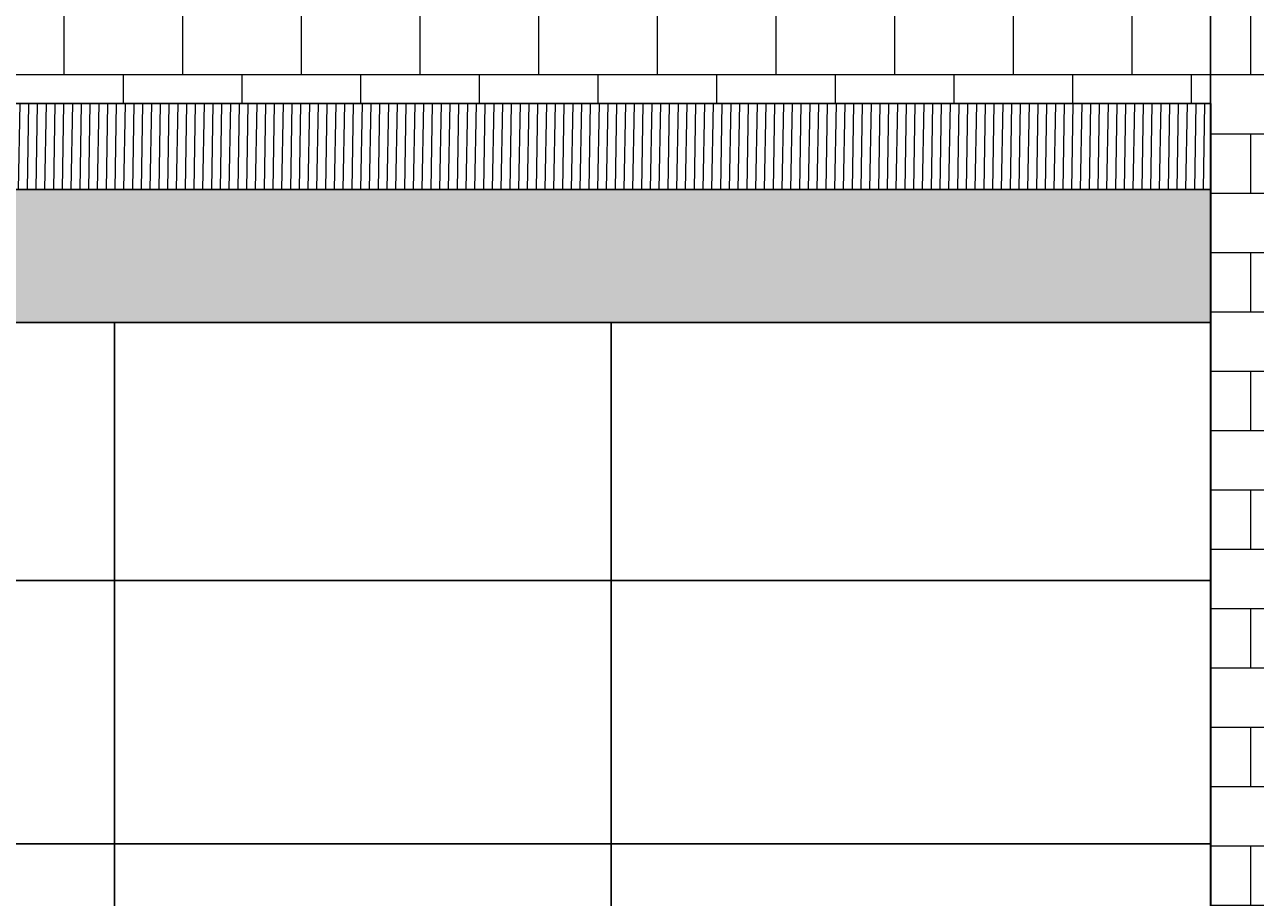
# Model space of a CAD drawing. Units: inches. Extents: x -26 to 776, y -22 to 650.
# Tile 6 of 62: x 98 to 222, y 67 to 155. Entities that reach past the tile are written whole.
import ezdxf

# ---------------------------------------------------------------- set-up
doc = ezdxf.new("R2010")
doc.units = ezdxf.units.IN
doc.header["$MEASUREMENT"] = 0
for name, color, linetype, lineweight in [('A-ANNO-DIMS', 2, 'Continuous', 18), ('A-DETL-PATT', 8, 'Continuous', 13), ('A-DOOR', 3, 'Continuous', 25), ('A-DOOR-PATT', 8, 'Continuous', 13), ('A-WALL-PATT', 8, 'Continuous', 13)]:
    doc.layers.add(name, color=color, linetype=linetype, lineweight=lineweight)
doc.styles.get("Standard").update_dxf_attribs({"font": 'arial.ttf'})
doc.dimstyles.get("Standard").update_dxf_attribs({"dimtxt": 0.5625, "dimasz": 0.18, "dimexe": 0.18, "dimexo": 0.0625, "dimgap": 0.09, "dimtad": 0, "dimtih": 1, "dimtoh": 1, "dimdec": 4, "dimzin": 0, "dimdsep": 46, "dimlunit": 4, "dimtxsty": 'Standard', "dimcen": 0.09, "dimadec": 0, "dimazin": 0, "dimtfac": 1, "dimtdec": 4, "dimtofl": 0, "dimtmove": 0, "dimatfit": 3, "dimfxl": 1, "dimtolj": 1, "dimtzin": 0, "dimarcsym": 0})

# ---------------------------------------------------------------- blocks, each defined once
blk = doc.blocks.new('*D14')
at = {"layer": 'A-ANNO-DIMS', "color": 0, "lineweight": -2, "transparency": 16777216}
for p, q in [((191.62, 613.27), (-25.48, 613.27)), ((-25.3, 613.09), (-25.3, 314.75)), ((-25.3, 15.66), (-25.3, 314)), ((11.04, 15.48), (-25.48, 15.48))]:
    blk.add_line(p, q, dxfattribs=at)
at = {"layer": 'A-ANNO-DIMS', "color": 0, "transparency": 16777216}
for points in [[(-25.33, 613.09), (-25.27, 613.09), (-25.3, 613.27)], [(-25.33, 15.66), (-25.27, 15.66), (-25.3, 15.48)]]:
    blk.add_solid(points, dxfattribs=at)
at = {"layer": 'Defpoints', "color": 0, "transparency": 16777216}
for p in [(-25.3, 613.27), (191.68, 613.27), (11.11, 15.48)]:
    blk.add_point(p, dxfattribs=at)
at = {"layer": 'A-ANNO-DIMS', "color": 0, "transparency": 16777216, "insert": (-25.3, 314.38), "char_height": 0.562, "attachment_point": 5}
blk.add_mtext('\\A1;597.8', dxfattribs=at)
blk = doc.blocks.new('*D22')
at = {"layer": 'A-ANNO-DIMS', "color": 0, "lineweight": -2, "transparency": 16777216}
for p, q in [((22.89, 15.33), (22.89, 649.86)), ((217.95, 15.54), (217.95, 649.86)), ((23.07, 649.68), (119.19, 649.68)), ((217.77, 649.68), (121.65, 649.68))]:
    blk.add_line(p, q, dxfattribs=at)
at = {"layer": 'A-ANNO-DIMS', "color": 0, "transparency": 16777216}
for points in [[(23.07, 649.71), (23.07, 649.65), (22.89, 649.68)], [(217.77, 649.71), (217.77, 649.65), (217.95, 649.68)]]:
    blk.add_solid(points, dxfattribs=at)
at = {"layer": 'Defpoints', "color": 0, "transparency": 16777216}
for p in [(217.95, 649.68), (22.89, 15.27), (217.95, 15.48)]:
    blk.add_point(p, dxfattribs=at)
at = {"layer": 'A-ANNO-DIMS', "color": 0, "transparency": 16777216, "insert": (120.42, 649.68), "char_height": 0.562, "attachment_point": 5}
blk.add_mtext('\\A1;195.06', dxfattribs=at)
blk = doc.blocks.new('*D37')
at = {"layer": 'A-ANNO-DIMS', "color": 0, "lineweight": -2, "transparency": 16777216}
for p, q in [((231.36, 159.48), (-25.48, 159.48)), ((-25.3, 159.3), (-25.3, 87.85)), ((-25.3, 15.66), (-25.3, 87.11)), ((217.89, 15.48), (-25.48, 15.48))]:
    blk.add_line(p, q, dxfattribs=at)
at = {"layer": 'A-ANNO-DIMS', "color": 0, "transparency": 16777216}
for points in [[(-25.33, 159.3), (-25.27, 159.3), (-25.3, 159.48)], [(-25.33, 15.66), (-25.27, 15.66), (-25.3, 15.48)]]:
    blk.add_solid(points, dxfattribs=at)
at = {"layer": 'Defpoints', "color": 0, "transparency": 16777216}
for p in [(-25.3, 159.48), (231.42, 159.48), (217.95, 15.48)]:
    blk.add_point(p, dxfattribs=at)
at = {"layer": 'A-ANNO-DIMS', "color": 0, "transparency": 16777216, "insert": (-25.3, 87.48), "char_height": 0.562, "attachment_point": 5}
blk.add_mtext('\\A1;144', dxfattribs=at)

msp = doc.modelspace()

# ---------------------------------------------------------------- hatches: boundary and pattern name
at = {"layer": 'A-DETL-PATT'}
h = msp.add_hatch(dxfattribs=at)
h.set_pattern_fill('ANSI31', color=256, scale=7.1, angle=44)
h.paths.add_polyline_path([(231.4249, 197.3298), (216.1056, 197.3298), (216.1056, 159.4824), (231.4249, 159.4824)])
h.paths.add_polyline_path([(236.4647, 197.3298), (231.4249, 197.3298), (231.4249, 159.4824), (276.1134, 159.4824), (276.1134, 171.4173), (236.4647, 171.4173)])
h.paths.add_polyline_path([(259.7413, 197.3298), (236.4647, 197.3298), (236.4647, 171.4173), (259.7413, 171.4173)], flags=17)
h.paths.add_polyline_path([(276.1134, 197.3298), (261.7413, 197.3298), (261.7413, 171.4173), (276.1134, 171.4173)], flags=17)
h.paths.add_polyline_path([(217.9529, 147.0781), (22.8891, 147.0781), (22.8891, 138.3844), (217.9529, 138.3844)])
h.paths.add_polyline_path([(285.0179, 152.3087), (285.0179, 159.4824), (231.4249, 159.4824), (240.1654, 144.8359), (280.6173, 144.8359)])
h.paths.add_polyline_path([(280.6173, 144.8359), (240.1654, 144.8359), (240.1654, 26.4239), (280.6173, 26.4239)])
h.paths.add_polyline_path([(274.6644, 134.8811), (274.6644, 34.0885), (245.7207, 34.0885), (245.7207, 134.8811)], flags=16)
h.paths.add_polyline_path([(285.0179, 303.3046), (236.4647, 303.3046), (236.4647, 294.4171), (285.0179, 294.4171)])
h.paths.add_polyline_path([(285.0179, 446.0063), (236.4647, 446.0063), (236.4647, 437.1188), (285.0179, 437.1188)])
at = {"layer": 'A-DOOR-PATT'}
h = msp.add_hatch(color=256, dxfattribs=at)
h.dxf.hatch_style = 1
h.paths.add_polyline_path([(217.9529, 138.3844), (22.8891, 138.3844), (22.8891, 124.9232), (217.9529, 124.9232)])
h.paths.add_polyline_path([(274.6644, 134.8811), (245.7207, 134.8811), (245.7207, 34.0885), (274.6644, 34.0885)])
at = {"layer": 'A-WALL-PATT'}
h = msp.add_hatch(dxfattribs=at)
h.set_pattern_fill('AR-B816', color=256, scale=0.75)
h.paths.add_polyline_path([(82.134, 209.6413), (11.1074, 209.6413), (11.1074, 159.4824), (82.134, 159.4824)])
h.paths.add_polyline_path([(231.4249, 209.6413), (209.091, 209.6413), (209.091, 159.4824), (214.1056, 159.4824), (214.1056, 199.3298), (231.4249, 199.3298)])
h.paths.add_polyline_path([(231.4249, 159.4824), (11.1074, 159.4824), (11.1074, 22.5014), (22.8891, 22.5014), (22.8891, 147.0781), (217.9529, 147.0781), (217.9529, 20.7937), (231.4249, 20.7937)])
h.paths.add_polyline_path([(285.0179, 152.3087), (280.6173, 144.8359), (280.6173, 26.4239), (240.1654, 26.4239), (240.1654, 144.8359), (231.4249, 159.4824), (231.4249, 20.7937), (285.0179, 20.7937)])

# ---------------------------------------------------------------- linework, layer by layer
at = {"layer": 'A-DOOR'}
for p, q in [((22.8891, 147.0781), (217.9529, 147.0781)), ((217.9529, 147.0781), (217.9529, 15.4824)), ((22.8891, 138.3844), (217.9529, 138.3844)), ((22.8891, 124.9232), (217.9529, 124.9232)), ((107.0893, 124.9232), (107.0893, 15.4824)), ((157.3287, 124.9232), (157.3287, 15.4824)), ((22.8891, 98.842), (217.9529, 98.842)), ((22.8891, 72.2), (217.9529, 72.2))]:
    msp.add_line(p, q, dxfattribs=at)

# ---------------------------------------------------------------- dimensions: what is measured, and where the dimension line sits
at = {"layer": 'A-ANNO-DIMS'}
dim = msp.add_linear_dim(base=(217.9529, 649.6763), p1=(22.8891, 15.2701), p2=(217.9529, 15.4824), dimstyle='Standard', override={"dimdec": 2, "dimlfac": 1, "dimrnd": 0, "dimzin": 0, "dimdsep": 46, "dimlunit": 2}, dxfattribs=at)
dim.commit()
dim.dimension.update_dxf_attribs({"geometry": '*D22', "text_midpoint": (120.421, 649.6763)})
for base, p1, p2, override, picture, middle in [((-25.2976, 613.2713), (11.1074, 15.4824), (191.6782, 613.2713), {"dimdec": 1, "dimlfac": 1, "dimrnd": 0, "dimzin": 0, "dimdsep": 46, "dimlunit": 2}, '*D14', (-25.2976, 314.3769)), ((-25.2976, 159.4824), (217.9529, 15.4824), (231.4249, 159.4824), {"dimdec": 0, "dimlfac": 1, "dimrnd": 0, "dimzin": 0, "dimdsep": 46, "dimlunit": 2}, '*D37', (-25.2976, 87.4824))]:
    dim = msp.add_linear_dim(base=base, p1=p1, p2=p2, angle=90, dimstyle='Standard', override=override, dxfattribs=at)
    dim.commit()
    dim.dimension.update_dxf_attribs({"geometry": picture, "text_midpoint": middle})

doc.saveas('drawing.dxf')
